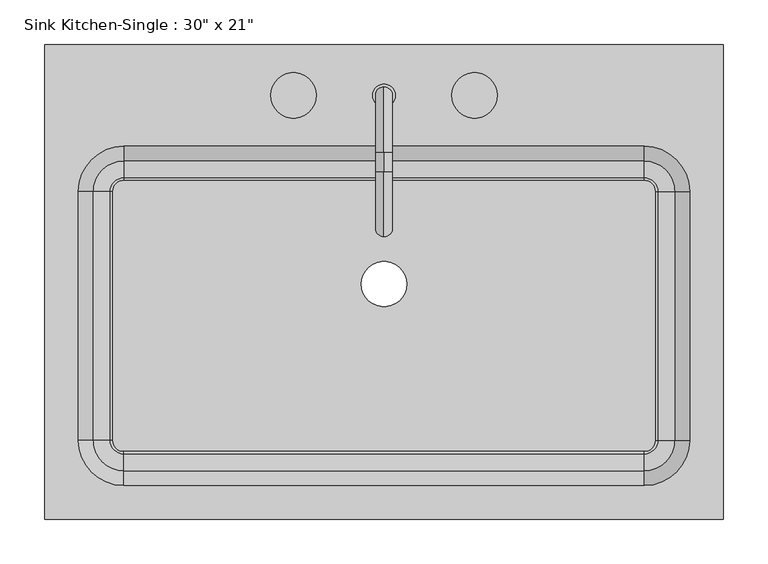
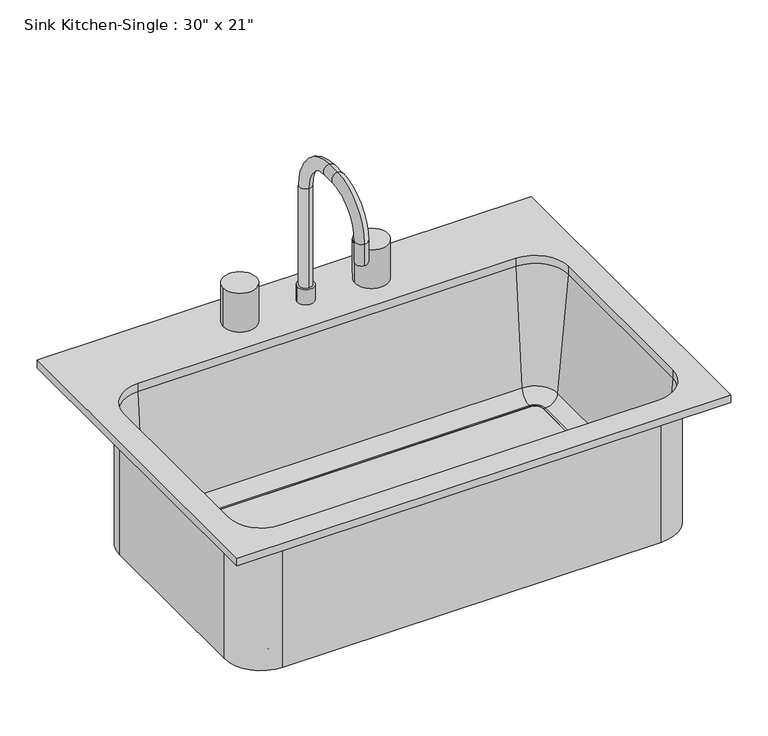
"""IFC4 building model written with IfcOpenShell, lengths in millimetres: flow terminal geometry."""

from ifc_helpers import new_model, si_unit, point, frame, frame_2d, origin, place, context, project, spatial, polyline, circle_curve, ellipse_curve, trimmed, segment, composite_curve, outline, extrude, source, transform, mapped, element, save
from ifc_brep_helpers import plane_surface, cylinder_surface, revolved_surface, advanced_brep


def flow_terminal_38af2918(model_context):
    return source(origin(), model_context, "Body", "SolidModel", [
        advanced_brep(
        [(396.6892406, 269.0454011, 927.1), (-365.3107594, 269.0454011, 927.1), (-365.3107594, -264.3545989, 927.1), (396.6892406, -264.3545989, 927.1), (307.7892406, 154.7454011, 927.1), (358.5892406, 103.9454011, 927.1), (358.5892406, -175.4545989, 927.1), (307.7892406, -226.2545989, 927.1), (-276.4107594, -226.2545989, 927.1), (-327.2107594, -175.4545989, 927.1), (-327.2107594, 103.9454011, 927.1), (-276.4107594, 154.7454011, 927.1), (396.6892406, 269.0454011, 914.4), (396.6892406, -264.3545989, 914.4), (-365.3107594, -264.3545989, 914.4), (-365.3107594, 269.0454011, 914.4), (364.9392406, 103.9454011, 914.4), (307.7892406, 161.0954011, 914.4), (-276.4107594, 161.0954011, 914.4), (-333.5607594, 103.9454011, 914.4), (-333.5607594, -175.4545989, 914.4), (-276.4107594, -232.6045989, 914.4), (307.7892406, -232.6045989, 914.4), (364.9392406, -175.4545989, 914.4), (307.7892406, 154.7454011, 914.4), (358.5892406, 103.9454011, 914.4), (358.5892406, -175.4545989, 914.4), (307.7892406, -226.2545989, 914.4), (-276.4107594, -226.2545989, 914.4), (-327.2107594, -175.4545989, 914.4), (-327.2107594, 103.9454011, 914.4), (-276.4107594, 154.7454011, 914.4), (364.9392406, 103.9454011, 698.5), (307.7892406, 161.0954011, 698.5), (320.4892406, 103.9454011, 698.5), (307.7892406, 116.6454011, 698.5), (320.4892406, 103.9454011, 708.025), (307.7892406, 116.6454011, 708.025), (323.0776588, 103.9454011, 708.025), (307.7892406, 119.2338193, 708.025), (342.0551678, 103.9454011, 725.4146831), (307.7892406, 138.2113283, 725.4146831), (364.9392406, -175.4545989, 698.5), (320.4892406, -175.4545989, 698.5), (320.4892406, -175.4545989, 708.025), (323.0776588, -175.4545989, 708.025), (342.0551678, -175.4545989, 725.4146831), (307.7892406, -232.6045989, 698.5), (307.7892406, -188.1545989, 698.5), (307.7892406, -188.1545989, 708.025), (307.7892406, -190.7430171, 708.025), (307.7892406, -209.7205261, 725.4146831), (-276.4107594, -232.6045989, 698.5), (-276.4107594, -188.1545989, 698.5), (-276.4107594, -188.1545989, 708.025), (-276.4107594, -190.7430171, 708.025), (-276.4107594, -209.7205261, 725.4146831), (-333.5607594, -175.4545989, 698.5), (-289.1107594, -175.4545989, 698.5), (-289.1107594, -175.4545989, 708.025), (-291.6991776, -175.4545989, 708.025), (-310.6766866, -175.4545989, 725.4146831), (-333.5607594, 103.9454011, 698.5), (-289.1107594, 103.9454011, 698.5), (-289.1107594, 103.9454011, 708.025), (-291.6991776, 103.9454011, 708.025), (-310.6766866, 103.9454011, 725.4146831), (-276.4107594, 161.0954011, 698.5), (-276.4107594, 116.6454011, 698.5), (-276.4107594, 116.6454011, 708.025), (-276.4107594, 119.2338193, 708.025), (-276.4107594, 138.2113283, 725.4146831)],
        [
            (0, 1),
            (1, 2),
            (2, 3),
            (3, 0),
            (4, 5, circle_curve(frame((307.7892406, 103.9454011, 927.1), z_axis=(0.0, 0.0, -1.0), x_axis=(1.0, 0.0, 0.0)), 50.8)),
            (5, 6),
            (6, 7, circle_curve(frame((307.7892406, -175.4545989, 927.1), z_axis=(0.0, 0.0, -1.0), x_axis=(1.0, 0.0, 0.0)), 50.8)),
            (7, 8),
            (8, 9, circle_curve(frame((-276.4107594, -175.4545989, 927.1), z_axis=(0.0, 0.0, -1.0), x_axis=(1.0, 0.0, 0.0)), 50.8)),
            (9, 10),
            (10, 11, circle_curve(frame((-276.4107594, 103.9454011, 927.1), z_axis=(0.0, 0.0, -1.0), x_axis=(1.0, 0.0, 0.0)), 50.8)),
            (11, 4),
            (12, 13),
            (13, 14),
            (14, 15),
            (15, 12),
            (16, 17, circle_curve(frame((307.7892406, 103.9454011, 914.4), z_axis=(0.0, 0.0, 1.0), x_axis=(0.0, 1.0, 0.0)), 57.15)),
            (17, 18),
            (18, 19, circle_curve(frame((-276.4107594, 103.9454011, 914.4), z_axis=(0.0, 0.0, 1.0), x_axis=(-1.0, 0.0, 0.0)), 57.15)),
            (19, 20),
            (20, 21, circle_curve(frame((-276.4107594, -175.4545989, 914.4), z_axis=(0.0, 0.0, 1.0), x_axis=(0.0, -1.0, 0.0)), 57.15)),
            (21, 22),
            (22, 23, circle_curve(frame((307.7892406, -175.4545989, 914.4), z_axis=(0.0, 0.0, 1.0), x_axis=(1.0, 0.0, 0.0)), 57.15)),
            (23, 16),
            (0, 12),
            (15, 1),
            (14, 2),
            (13, 3),
            (4, 24),
            (24, 25, circle_curve(frame((307.7892406, 103.9454011, 914.4), z_axis=(0.0, 0.0, -1.0), x_axis=(1.0, 0.0, 0.0)), 50.8)),
            (25, 5),
            (25, 26),
            (26, 6),
            (26, 27, circle_curve(frame((307.7892406, -175.4545989, 914.4), z_axis=(0.0, 0.0, -1.0), x_axis=(1.0, 0.0, 0.0)), 50.8)),
            (27, 7),
            (27, 28),
            (28, 8),
            (28, 29, circle_curve(frame((-276.4107594, -175.4545989, 914.4), z_axis=(0.0, 0.0, -1.0), x_axis=(1.0, 0.0, 0.0)), 50.8)),
            (29, 9),
            (29, 30),
            (30, 10),
            (30, 31, circle_curve(frame((-276.4107594, 103.9454011, 914.4), z_axis=(0.0, 0.0, -1.0), x_axis=(1.0, 0.0, 0.0)), 50.8)),
            (31, 11),
            (31, 24),
            (32, 33, circle_curve(frame((307.7892406, 103.9454011, 698.5), z_axis=(0.0, 0.0, 1.0), x_axis=(0.0, 1.0, 0.0)), 57.15)),
            (33, 17),
            (16, 32),
            (32, 34),
            (34, 35, circle_curve(frame((307.7892406, 103.9454011, 698.5), z_axis=(0.0, 0.0, 1.0), x_axis=(0.0, 1.0, 0.0)), 12.7)),
            (35, 33),
            (34, 36),
            (36, 37, circle_curve(frame((307.7892406, 103.9454011, 708.025), z_axis=(0.0, 0.0, 1.0), x_axis=(0.0, 1.0, 0.0)), 12.7)),
            (37, 35),
            (36, 38),
            (38, 39, circle_curve(frame((307.7892406, 103.9454011, 708.025), z_axis=(0.0, 0.0, 1.0), x_axis=(0.0, 1.0, 0.0)), 15.2884182)),
            (39, 37),
            (38, 40, circle_curve(frame((323.0776588, 103.9454011, 727.075), z_axis=(0.0, -1.0, 0.0), x_axis=(1.0, 0.0, 0.0)), 19.05)),
            (40, 41, circle_curve(frame((307.7892406, 103.9454011, 725.4146831), z_axis=(0.0, 0.0, 1.0), x_axis=(0.0, 1.0, 0.0)), 34.2659272)),
            (41, 39, circle_curve(frame((307.7892406, 119.2338193, 727.075), z_axis=(-1.0, 0.0, 0.0), x_axis=(0.0, 1.0, 0.0)), 19.05)),
            (40, 25),
            (24, 41),
            (23, 42),
            (42, 32),
            (42, 43),
            (43, 34),
            (43, 44),
            (44, 36),
            (44, 45),
            (45, 38),
            (45, 46, circle_curve(frame((323.0776588, -175.4545989, 727.075), z_axis=(0.0, -1.0, 0.0), x_axis=(1.0, 0.0, 0.0)), 19.05)),
            (46, 40),
            (46, 26),
            (22, 47),
            (47, 42, circle_curve(frame((307.7892406, -175.4545989, 698.5), z_axis=(0.0, 0.0, 1.0), x_axis=(1.0, 0.0, 0.0)), 57.15)),
            (47, 48),
            (48, 43, circle_curve(frame((307.7892406, -175.4545989, 698.5), z_axis=(0.0, 0.0, 1.0), x_axis=(1.0, 0.0, 0.0)), 12.7)),
            (48, 49),
            (49, 44, circle_curve(frame((307.7892406, -175.4545989, 708.025), z_axis=(0.0, 0.0, 1.0), x_axis=(1.0, 0.0, 0.0)), 12.7)),
            (49, 50),
            (50, 45, circle_curve(frame((307.7892406, -175.4545989, 708.025), z_axis=(0.0, 0.0, 1.0), x_axis=(1.0, 0.0, 0.0)), 15.2884182)),
            (50, 51, circle_curve(frame((307.7892406, -190.7430171, 727.075), z_axis=(-1.0, 0.0, 0.0), x_axis=(0.0, -1.0, 0.0)), 19.05)),
            (51, 46, circle_curve(frame((307.7892406, -175.4545989, 725.4146831), z_axis=(0.0, 0.0, 1.0), x_axis=(1.0, 0.0, 0.0)), 34.2659272)),
            (51, 27),
            (21, 52),
            (52, 47),
            (52, 53),
            (53, 48),
            (53, 54),
            (54, 49),
            (54, 55),
            (55, 50),
            (55, 56, circle_curve(frame((-276.4107594, -190.7430171, 727.075), z_axis=(-1.0, 0.0, 0.0), x_axis=(0.0, -1.0, 0.0)), 19.05)),
            (56, 51),
            (56, 28),
            (20, 57),
            (57, 52, circle_curve(frame((-276.4107594, -175.4545989, 698.5), z_axis=(0.0, 0.0, 1.0), x_axis=(0.0, -1.0, 0.0)), 57.15)),
            (57, 58),
            (58, 53, circle_curve(frame((-276.4107594, -175.4545989, 698.5), z_axis=(0.0, 0.0, 1.0), x_axis=(0.0, -1.0, 0.0)), 12.7)),
            (58, 59),
            (59, 54, circle_curve(frame((-276.4107594, -175.4545989, 708.025), z_axis=(0.0, 0.0, 1.0), x_axis=(0.0, -1.0, 0.0)), 12.7)),
            (59, 60),
            (60, 55, circle_curve(frame((-276.4107594, -175.4545989, 708.025), z_axis=(0.0, 0.0, 1.0), x_axis=(0.0, -1.0, 0.0)), 15.2884182)),
            (60, 61, circle_curve(frame((-291.6991776, -175.4545989, 727.075), z_axis=(0.0, 1.0, 0.0), x_axis=(-1.0, 0.0, 0.0)), 19.05)),
            (61, 56, circle_curve(frame((-276.4107594, -175.4545989, 725.4146831), z_axis=(0.0, 0.0, 1.0), x_axis=(0.0, -1.0, 0.0)), 34.2659272)),
            (61, 29),
            (19, 62),
            (62, 57),
            (62, 63),
            (63, 58),
            (63, 64),
            (64, 59),
            (64, 65),
            (65, 60),
            (65, 66, circle_curve(frame((-291.6991776, 103.9454011, 727.075), z_axis=(0.0, 1.0, 0.0), x_axis=(-1.0, 0.0, 0.0)), 19.05)),
            (66, 61),
            (66, 30),
            (18, 67),
            (67, 62, circle_curve(frame((-276.4107594, 103.9454011, 698.5), z_axis=(0.0, 0.0, 1.0), x_axis=(-1.0, 0.0, 0.0)), 57.15)),
            (67, 68),
            (68, 63, circle_curve(frame((-276.4107594, 103.9454011, 698.5), z_axis=(0.0, 0.0, 1.0), x_axis=(-1.0, 0.0, 0.0)), 12.7)),
            (68, 69),
            (69, 64, circle_curve(frame((-276.4107594, 103.9454011, 708.025), z_axis=(0.0, 0.0, 1.0), x_axis=(-1.0, 0.0, 0.0)), 12.7)),
            (69, 70),
            (70, 65, circle_curve(frame((-276.4107594, 103.9454011, 708.025), z_axis=(0.0, 0.0, 1.0), x_axis=(-1.0, 0.0, 0.0)), 15.2884182)),
            (70, 71, circle_curve(frame((-276.4107594, 119.2338193, 727.075), z_axis=(1.0, 0.0, 0.0), x_axis=(0.0, 1.0, 0.0)), 19.05)),
            (71, 66, circle_curve(frame((-276.4107594, 103.9454011, 725.4146831), z_axis=(0.0, 0.0, 1.0), x_axis=(-1.0, 0.0, 0.0)), 34.2659272)),
            (71, 31),
            (33, 67),
            (35, 68),
            (37, 69),
            (39, 70),
            (41, 71),
        ],
        [
            plane_surface(frame((-365.3107594, 269.0454011, 927.1), z_axis=(0.0, 0.0, 1.0), x_axis=(-1.0, 0.0, 0.0))),
            plane_surface(frame((-365.3107594, 269.0454011, 914.4), z_axis=(0.0, 0.0, -1.0), x_axis=(1.0, 0.0, 0.0))),
            plane_surface(frame((396.6892406, 269.0454011, 927.1), z_axis=(0.0, 1.0, 0.0), x_axis=(0.0, 0.0, -1.0))),
            plane_surface(frame((-365.3107594, 269.0454011, 927.1), z_axis=(-1.0, 0.0, 0.0), x_axis=(0.0, 0.0, -1.0))),
            plane_surface(frame((-365.3107594, -264.3545989, 927.1), z_axis=(0.0, -1.0, 0.0), x_axis=(0.0, 0.0, -1.0))),
            plane_surface(frame((396.6892406, -264.3545989, 927.1), z_axis=(1.0, 0.0, 0.0), x_axis=(0.0, 0.0, -1.0))),
            revolved_surface(polyline([(358.58924060000004, 103.9454011, 914.4), (358.58924060000004, 103.9454011, 927.1)]), (307.7892406, 103.9454011, 0.0), (0.0, 0.0, -1.0)),
            plane_surface(frame((358.5892406, 103.9454011, 927.1), z_axis=(-1.0, 0.0, 0.0), x_axis=(0.0, 0.0, -1.0))),
            revolved_surface(polyline([(358.58924060000004, -175.4545989, 914.4), (358.58924060000004, -175.4545989, 927.1)]), (307.7892406, -175.4545989, 0.0), (0.0, 0.0, -1.0)),
            plane_surface(frame((307.7892406, -226.2545989, 927.1), z_axis=(0.0, 1.0, 0.0), x_axis=(0.0, 0.0, -1.0))),
            revolved_surface(polyline([(-225.6107594, -175.4545989, 914.4), (-225.6107594, -175.4545989, 927.1)]), (-276.4107594, -175.4545989, 0.0), (0.0, 0.0, -1.0)),
            plane_surface(frame((-327.2107594, -175.4545989, 927.1), z_axis=(1.0, 0.0, 0.0), x_axis=(0.0, 0.0, -1.0))),
            revolved_surface(polyline([(-225.6107594, 103.9454011, 914.4), (-225.6107594, 103.9454011, 927.1)]), (-276.4107594, 103.9454011, 0.0), (0.0, 0.0, -1.0)),
            plane_surface(frame((-276.4107594, 154.7454011, 927.1), z_axis=(0.0, -1.0, 0.0), x_axis=(0.0, 0.0, -1.0))),
            cylinder_surface(frame((307.7892406, 103.9454011, 0.0), z_axis=(0.0, 0.0, -1.0), x_axis=(0.0, 1.0, 0.0)), 57.15),
            plane_surface(frame((307.7892406, 103.9454011, 698.5), z_axis=(0.0, 0.0, -1.0), x_axis=(0.0, 1.0, 0.0))),
            revolved_surface(polyline([(307.7892406, 116.6454011, 698.5), (307.7892406, 116.6454011, 708.025)]), (307.7892406, 103.9454011, 0.0), (0.0, 0.0, -1.0)),
            plane_surface(frame((307.7892406, 103.9454011, 708.025), z_axis=(0.0, 0.0, 1.0), x_axis=(0.0, 1.0, 0.0))),
            revolved_surface(trimmed(ellipse_curve(frame((307.7892406, 119.2338193, 727.075), z_axis=(1.0, 0.0, 0.0), x_axis=(0.0, 1.0, 0.0)), 19.05, 19.05), [point((307.7892406, 119.2338193, 708.025))], [point((307.7892406, 138.2113283, 725.4146831))], True, "CARTESIAN"), (307.7892406, 103.9454011, 0.0), (0.0, 0.0, -1.0)),
            revolved_surface(polyline([(307.7892406, 138.2113283, 725.4146831), (307.7892406, 154.7454011, 914.4)]), (307.7892406, 103.9454011, 0.0), (0.0, 0.0, -1.0)),
            plane_surface(frame((364.9392406, 103.9454011, 914.4), z_axis=(1.0, 0.0, 0.0), x_axis=(0.0, -1.0, 0.0))),
            plane_surface(frame((364.9392406, 103.9454011, 698.5), z_axis=(0.0, 0.0, -1.0), x_axis=(0.0, -1.0, 0.0))),
            plane_surface(frame((320.4892406, 103.9454011, 698.5), z_axis=(-1.0, 0.0, 0.0), x_axis=(0.0, -1.0, 0.0))),
            plane_surface(frame((320.4892406, 103.9454011, 708.025), z_axis=(0.0, 0.0, 1.0), x_axis=(0.0, -1.0, 0.0))),
            revolved_surface(polyline([(342.1276588, -175.45459889999998, 727.075), (342.1276588, 103.9454011, 727.075)]), (323.0776588, 103.9454011, 727.075), (0.0, -1.0, 0.0)),
            plane_surface(frame((342.0551678, 103.9454011, 725.4146831), z_axis=(-0.9961946980917442, 0.0, 0.08715574274767306), x_axis=(0.0, -1.0, 0.0))),
            cylinder_surface(frame((307.7892406, -175.4545989, 0.0), z_axis=(0.0, 0.0, -1.0), x_axis=(1.0, 0.0, 0.0)), 57.15),
            plane_surface(frame((307.7892406, -175.4545989, 698.5), z_axis=(0.0, 0.0, -1.0), x_axis=(1.0, 0.0, 0.0))),
            revolved_surface(polyline([(320.4892406, -175.4545989, 698.5), (320.4892406, -175.4545989, 708.025)]), (307.7892406, -175.4545989, 0.0), (0.0, 0.0, -1.0)),
            plane_surface(frame((307.7892406, -175.4545989, 708.025), z_axis=(0.0, 0.0, 1.0), x_axis=(1.0, 0.0, 0.0))),
            revolved_surface(trimmed(ellipse_curve(frame((323.0776588, -175.4545989, 727.075), z_axis=(0.0, -1.0, 0.0), x_axis=(1.0, 0.0, 0.0)), 19.05, 19.05), [point((323.0776588, -175.4545989, 708.025))], [point((342.0551678, -175.4545989, 725.4146831))], True, "CARTESIAN"), (307.7892406, -175.4545989, 0.0), (0.0, 0.0, -1.0)),
            revolved_surface(polyline([(342.0551678, -175.4545989, 725.4146831), (358.5892406, -175.4545989, 914.4)]), (307.7892406, -175.4545989, 0.0), (0.0, 0.0, -1.0)),
            plane_surface(frame((307.7892406, -232.6045989, 914.4), z_axis=(0.0, -1.0, 0.0), x_axis=(-1.0, 0.0, 0.0))),
            plane_surface(frame((307.7892406, -232.6045989, 698.5), z_axis=(0.0, 0.0, -1.0), x_axis=(-1.0, 0.0, 0.0))),
            plane_surface(frame((307.7892406, -188.1545989, 698.5), z_axis=(0.0, 1.0, 0.0), x_axis=(-1.0, 0.0, 0.0))),
            plane_surface(frame((307.7892406, -188.1545989, 708.025), z_axis=(0.0, 0.0, 1.0), x_axis=(-1.0, 0.0, 0.0))),
            revolved_surface(polyline([(-276.4107594, -209.79301710000001, 727.075), (307.7892406, -209.79301710000001, 727.075)]), (307.7892406, -190.7430171, 727.075), (-1.0, 0.0, 0.0)),
            plane_surface(frame((307.7892406, -209.7205261, 725.4146831), z_axis=(0.0, 0.9961946980917442, 0.08715574274767306), x_axis=(-1.0, 0.0, 0.0))),
            cylinder_surface(frame((-276.4107594, -175.4545989, 0.0), z_axis=(0.0, 0.0, -1.0), x_axis=(0.0, -1.0, 0.0)), 57.15),
            plane_surface(frame((-276.4107594, -175.4545989, 698.5), z_axis=(0.0, 0.0, -1.0), x_axis=(0.0, -1.0, 0.0))),
            revolved_surface(polyline([(-276.4107594, -188.1545989, 698.5), (-276.4107594, -188.1545989, 708.025)]), (-276.4107594, -175.4545989, 0.0), (0.0, 0.0, -1.0)),
            plane_surface(frame((-276.4107594, -175.4545989, 708.025), z_axis=(0.0, 0.0, 1.0), x_axis=(0.0, -1.0, 0.0))),
            revolved_surface(trimmed(ellipse_curve(frame((-276.4107594, -190.7430171, 727.075), z_axis=(-1.0, 0.0, 0.0), x_axis=(0.0, -1.0, 0.0)), 19.05, 19.05), [point((-276.4107594, -190.7430171, 708.025))], [point((-276.4107594, -209.7205261, 725.4146831))], True, "CARTESIAN"), (-276.4107594, -175.4545989, 0.0), (0.0, 0.0, -1.0)),
            revolved_surface(polyline([(-276.4107594, -209.7205261, 725.4146831), (-276.4107594, -226.2545989, 914.4)]), (-276.4107594, -175.4545989, 0.0), (0.0, 0.0, -1.0)),
            plane_surface(frame((-333.5607594, -175.4545989, 914.4), z_axis=(-1.0, 0.0, 0.0), x_axis=(0.0, 1.0, 0.0))),
            plane_surface(frame((-333.5607594, -175.4545989, 698.5), z_axis=(0.0, 0.0, -1.0), x_axis=(0.0, 1.0, 0.0))),
            plane_surface(frame((-289.1107594, -175.4545989, 698.5), z_axis=(1.0, 0.0, 0.0), x_axis=(0.0, 1.0, 0.0))),
            plane_surface(frame((-289.1107594, -175.4545989, 708.025), z_axis=(0.0, 0.0, 1.0), x_axis=(0.0, 1.0, 0.0))),
            revolved_surface(polyline([(-310.7491776, 103.94540109999997, 727.075), (-310.7491776, -175.4545989, 727.075)]), (-291.6991776, -175.4545989, 727.075), (0.0, 1.0, 0.0)),
            plane_surface(frame((-310.6766866, -175.4545989, 725.4146831), z_axis=(0.9961946980917442, 0.0, 0.08715574274767306), x_axis=(0.0, 1.0, 0.0))),
            cylinder_surface(frame((-276.4107594, 103.9454011, 0.0), z_axis=(0.0, 0.0, -1.0), x_axis=(-1.0, 0.0, 0.0)), 57.15),
            plane_surface(frame((-276.4107594, 103.9454011, 698.5), z_axis=(0.0, 0.0, -1.0), x_axis=(-1.0, 0.0, 0.0))),
            revolved_surface(polyline([(-289.1107594, 103.9454011, 698.5), (-289.1107594, 103.9454011, 708.025)]), (-276.4107594, 103.9454011, 0.0), (0.0, 0.0, -1.0)),
            plane_surface(frame((-276.4107594, 103.9454011, 708.025), z_axis=(0.0, 0.0, 1.0), x_axis=(-1.0, 0.0, 0.0))),
            revolved_surface(trimmed(ellipse_curve(frame((-291.6991776, 103.9454011, 727.075), z_axis=(0.0, 1.0, 0.0), x_axis=(-1.0, 0.0, 0.0)), 19.05, 19.05), [point((-291.6991776, 103.9454011, 708.025))], [point((-310.6766866, 103.9454011, 725.4146831))], True, "CARTESIAN"), (-276.4107594, 103.9454011, 0.0), (0.0, 0.0, -1.0)),
            revolved_surface(polyline([(-310.6766866, 103.9454011, 725.4146831), (-327.2107594, 103.9454011, 914.4)]), (-276.4107594, 103.9454011, 0.0), (0.0, 0.0, -1.0)),
            plane_surface(frame((-276.4107594, 161.0954011, 914.4), z_axis=(0.0, 1.0, 0.0), x_axis=(1.0, 0.0, 0.0))),
            plane_surface(frame((-276.4107594, 161.0954011, 698.5), z_axis=(0.0, 0.0, -1.0), x_axis=(1.0, 0.0, 0.0))),
            plane_surface(frame((-276.4107594, 116.6454011, 698.5), z_axis=(0.0, -1.0, 0.0), x_axis=(1.0, 0.0, 0.0))),
            plane_surface(frame((-276.4107594, 116.6454011, 708.025), z_axis=(0.0, 0.0, 1.0), x_axis=(1.0, 0.0, 0.0))),
            revolved_surface(polyline([(307.7892406, 138.2838193, 727.075), (-276.4107594, 138.2838193, 727.075)]), (-276.4107594, 119.2338193, 727.075), (1.0, 0.0, 0.0)),
            plane_surface(frame((-276.4107594, 138.2113283, 725.4146831), z_axis=(0.0, -0.9961946980917442, 0.08715574274767306), x_axis=(1.0, 0.0, 0.0))),
        ],
        [
            (0, [[1, 2, 3, 4], [5, 6, 7, 8, 9, 10, 11, 12]]),
            (1, [[13, 14, 15, 16], [17, 18, 19, 20, 21, 22, 23, 24]]),
            (2, [[-1, 25, -16, 26]]),
            (3, [[-2, -26, -15, 27]]),
            (4, [[-3, -27, -14, 28]]),
            (5, [[-4, -28, -13, -25]]),
            (6, [[-5, 29, 30, 31]]),
            (7, [[-6, -31, 32, 33]]),
            (8, [[-7, -33, 34, 35]]),
            (9, [[-8, -35, 36, 37]]),
            (10, [[-9, -37, 38, 39]]),
            (11, [[-10, -39, 40, 41]]),
            (12, [[-11, -41, 42, 43]]),
            (13, [[-12, -43, 44, -29]]),
            (14, [[45, 46, -17, 47]]),
            (15, [[-45, 48, 49, 50]]),
            (16, [[-49, 51, 52, 53]]),
            (17, [[-52, 54, 55, 56]]),
            (18, [[-55, 57, 58, 59]]),
            (19, [[-58, 60, -30, 61]]),
            (20, [[-47, -24, 62, 63]]),
            (21, [[-48, -63, 64, 65]]),
            (22, [[-51, -65, 66, 67]]),
            (23, [[-54, -67, 68, 69]]),
            (24, [[-57, -69, 70, 71]]),
            (25, [[-60, -71, 72, -32]]),
            (26, [[-62, -23, 73, 74]]),
            (27, [[-64, -74, 75, 76]]),
            (28, [[-66, -76, 77, 78]]),
            (29, [[-68, -78, 79, 80]]),
            (30, [[-70, -80, 81, 82]]),
            (31, [[-72, -82, 83, -34]]),
            (32, [[-73, -22, 84, 85]]),
            (33, [[-75, -85, 86, 87]]),
            (34, [[-77, -87, 88, 89]]),
            (35, [[-79, -89, 90, 91]]),
            (36, [[-81, -91, 92, 93]]),
            (37, [[-83, -93, 94, -36]]),
            (38, [[-84, -21, 95, 96]]),
            (39, [[-86, -96, 97, 98]]),
            (40, [[-88, -98, 99, 100]]),
            (41, [[-90, -100, 101, 102]]),
            (42, [[-92, -102, 103, 104]]),
            (43, [[-94, -104, 105, -38]]),
            (44, [[-95, -20, 106, 107]]),
            (45, [[-97, -107, 108, 109]]),
            (46, [[-99, -109, 110, 111]]),
            (47, [[-101, -111, 112, 113]]),
            (48, [[-103, -113, 114, 115]]),
            (49, [[-105, -115, 116, -40]]),
            (50, [[-106, -19, 117, 118]]),
            (51, [[-108, -118, 119, 120]]),
            (52, [[-110, -120, 121, 122]]),
            (53, [[-112, -122, 123, 124]]),
            (54, [[-114, -124, 125, 126]]),
            (55, [[-116, -126, 127, -42]]),
            (56, [[-46, 128, -117, -18]]),
            (57, [[-50, 129, -119, -128]]),
            (58, [[-53, 130, -121, -129]]),
            (59, [[-56, 131, -123, -130]]),
            (60, [[-59, 132, -125, -131]]),
            (61, [[-61, -44, -127, -132]]),
        ],
    ),
        advanced_brep(
        [(2.9892406, 211.8954011, 927.1), (28.3892406, 211.8954011, 927.1), (15.6892406, 221.4204011, 1114.425), (15.6892406, 202.3704011, 1114.425), (15.6892406, 202.3704011, 952.5), (15.6892406, 221.4204011, 952.5), (15.6892406, 148.3954011, 1187.45), (15.6892406, 148.3954011, 1168.4), (15.6892406, 126.1704011, 1187.45), (15.6892406, 126.1704011, 1168.4), (15.6892406, 53.1454011, 1114.425), (15.6892406, 72.1954011, 1114.425), (15.6892406, 53.1454011, 1079.5), (15.6892406, 72.1954011, 1079.5), (2.9892406, 211.8954011, 952.5), (28.3892406, 211.8954011, 952.5)],
        [
            (0, 1, circle_curve(frame((15.6892406, 211.8954011, 927.1), z_axis=(0.0, 0.0, -1.0), x_axis=(1.0, 0.0, 0.0)), 12.7)),
            (1, 0, circle_curve(frame((15.6892406, 211.8954011, 927.1), z_axis=(0.0, 0.0, -1.0), x_axis=(1.0, 0.0, 0.0)), 12.7)),
            (2, 3, circle_curve(frame((15.6892406, 211.8954011, 1114.425), z_axis=(0.0, 0.0, -1.0), x_axis=(0.0, -1.0, 0.0)), 9.525)),
            (3, 4),
            (4, 5, circle_curve(frame((15.6892406, 211.8954011, 952.5), z_axis=(0.0, 0.0, 1.0), x_axis=(0.0, -1.0, 0.0)), 9.525)),
            (5, 2),
            (3, 2, circle_curve(frame((15.6892406, 211.8954011, 1114.425), z_axis=(0.0, 0.0, -1.0), x_axis=(0.0, -1.0, 0.0)), 9.525)),
            (5, 4, circle_curve(frame((15.6892406, 211.8954011, 952.5), z_axis=(0.0, 0.0, 1.0), x_axis=(0.0, -1.0, 0.0)), 9.525)),
            (2, 6, circle_curve(frame((15.6892406, 148.3954011, 1114.425), z_axis=(1.0, 0.0, 0.0), x_axis=(0.0, 1.0, 0.0)), 73.025)),
            (6, 7, circle_curve(frame((15.6892406, 148.3954011, 1177.925), z_axis=(0.0, 1.0, 0.0), x_axis=(0.0, 0.0, -1.0)), 9.525)),
            (7, 3, circle_curve(frame((15.6892406, 148.3954011, 1114.425), z_axis=(-1.0, 0.0, 0.0), x_axis=(0.0, 1.0, 0.0)), 53.975)),
            (7, 6, circle_curve(frame((15.6892406, 148.3954011, 1177.925), z_axis=(0.0, 1.0, 0.0), x_axis=(0.0, 0.0, -1.0)), 9.525)),
            (6, 8),
            (8, 9, circle_curve(frame((15.6892406, 126.1704011, 1177.925), z_axis=(0.0, 1.0, 0.0), x_axis=(0.0, 0.0, -1.0)), 9.525)),
            (9, 7),
            (9, 8, circle_curve(frame((15.6892406, 126.1704011, 1177.925), z_axis=(0.0, 1.0, 0.0), x_axis=(0.0, 0.0, -1.0)), 9.525)),
            (8, 10, circle_curve(frame((15.6892406, 126.1704011, 1114.425), z_axis=(1.0, 0.0, 0.0), x_axis=(0.0, 0.0, 1.0)), 73.025)),
            (10, 11, circle_curve(frame((15.6892406, 62.6704011, 1114.425), z_axis=(0.0, 0.0, 1.0), x_axis=(0.0, 1.0, 0.0)), 9.525)),
            (11, 9, circle_curve(frame((15.6892406, 126.1704011, 1114.425), z_axis=(-1.0, 0.0, 0.0), x_axis=(0.0, 0.0, 1.0)), 53.975)),
            (11, 10, circle_curve(frame((15.6892406, 62.6704011, 1114.425), z_axis=(0.0, 0.0, 1.0), x_axis=(0.0, 1.0, 0.0)), 9.525)),
            (12, 13, circle_curve(frame((15.6892406, 62.6704011, 1079.5), z_axis=(0.0, 0.0, -1.0), x_axis=(0.0, 1.0, 0.0)), 9.525)),
            (13, 12, circle_curve(frame((15.6892406, 62.6704011, 1079.5), z_axis=(0.0, 0.0, -1.0), x_axis=(0.0, 1.0, 0.0)), 9.525)),
            (10, 12),
            (13, 11),
            (14, 15, circle_curve(frame((15.6892406, 211.8954011, 952.5), z_axis=(0.0, 0.0, 1.0), x_axis=(1.0, 0.0, 0.0)), 12.7)),
            (15, 14, circle_curve(frame((15.6892406, 211.8954011, 952.5), z_axis=(0.0, 0.0, 1.0), x_axis=(1.0, 0.0, 0.0)), 12.7)),
            (14, 0),
            (1, 15),
        ],
        [
            plane_surface(frame((15.6892406, 202.3704011, 927.1), z_axis=(0.0, 0.0, -1.0), x_axis=(1.0, 0.0, 0.0))),
            cylinder_surface(frame((15.6892406, 211.8954011, 927.1), z_axis=(0.0, 0.0, -1.0), x_axis=(0.0, -1.0, 0.0)), 9.525),
            revolved_surface(trimmed(ellipse_curve(frame((15.6892406, 211.8954011, 1114.425), z_axis=(0.0, 0.0, -1.0), x_axis=(0.0, -1.0, 0.0)), 9.525, 9.525), [point((15.6892406, 221.4204011, 1114.425))], [point((15.6892406, 202.3704011, 1114.425))], True, "CARTESIAN"), (15.6892406, 148.3954011, 1114.425), (1.0, 0.0, 0.0)),
            revolved_surface(trimmed(ellipse_curve(frame((15.6892406, 211.8954011, 1114.425), z_axis=(0.0, 0.0, -1.0), x_axis=(0.0, -1.0, 0.0)), 9.525, 9.525), [point((15.6892406, 202.3704011, 1114.425))], [point((15.6892406, 221.4204011, 1114.425))], True, "CARTESIAN"), (15.6892406, 148.3954011, 1114.425), (1.0, 0.0, 0.0)),
            cylinder_surface(frame((15.6892406, 148.3954011, 1177.925), z_axis=(0.0, 1.0, 0.0), x_axis=(0.0, 0.0, -1.0)), 9.525),
            revolved_surface(trimmed(ellipse_curve(frame((15.6892406, 126.1704011, 1177.925), z_axis=(0.0, 1.0, 0.0), x_axis=(0.0, 0.0, -1.0)), 9.525, 9.525), [point((15.6892406, 126.1704011, 1187.45))], [point((15.6892406, 126.1704011, 1168.4))], True, "CARTESIAN"), (15.6892406, 126.1704011, 1114.425), (1.0, 0.0, 0.0)),
            revolved_surface(trimmed(ellipse_curve(frame((15.6892406, 126.1704011, 1177.925), z_axis=(0.0, 1.0, 0.0), x_axis=(0.0, 0.0, -1.0)), 9.525, 9.525), [point((15.6892406, 126.1704011, 1168.4))], [point((15.6892406, 126.1704011, 1187.45))], True, "CARTESIAN"), (15.6892406, 126.1704011, 1114.425), (1.0, 0.0, 0.0)),
            plane_surface(frame((15.6892406, 53.1454011, 1079.5), z_axis=(0.0, 0.0, -1.0), x_axis=(-1.0, 0.0, 0.0))),
            cylinder_surface(frame((15.6892406, 62.6704011, 1114.425), z_axis=(0.0, 0.0, 1.0), x_axis=(0.0, 1.0, 0.0)), 9.525),
            plane_surface(frame((28.3892406, 211.8954011, 952.5), z_axis=(0.0, 0.0, 1.0), x_axis=(0.0, 1.0, 0.0))),
            cylinder_surface(frame((15.6892406, 211.8954011, 927.1), z_axis=(0.0, 0.0, 1.0), x_axis=(1.0, 0.0, 0.0)), 12.7),
        ],
        [
            (0, [[1, 2]]),
            (1, [[3, 4, 5, 6]]),
            (1, [[7, -6, 8, -4]]),
            (2, [[-3, 9, 10, 11]]),
            (3, [[-7, -11, 12, -9]]),
            (4, [[-10, 13, 14, 15]]),
            (4, [[-12, -15, 16, -13]]),
            (5, [[-14, 17, 18, 19]]),
            (6, [[-16, -19, 20, -17]]),
            (7, [[21, 22]]),
            (8, [[-18, 23, -22, 24]]),
            (8, [[-20, -24, -21, -23]]),
            (9, [[25, 26], [-5, -8]]),
            (10, [[-25, 27, -2, 28]]),
            (10, [[-26, -28, -1, -27]]),
        ],
    ),
        extrude(outline(composite_curve([segment(trimmed(circle_curve(frame_2d((-85.9107594, 211.8954011)), 25.4), [point((-111.3107594, 211.8954011))], [point((-60.5107594, 211.8954011))], False, "CARTESIAN"), True, "CONTINUOUS"), segment(trimmed(circle_curve(frame_2d((-85.9107594, 211.8954011)), 25.4), [point((-60.5107594, 211.8954011))], [point((-111.3107594, 211.8954011))], False, "CARTESIAN"), True, "CONTINUOUS")], self_intersect=False)), frame((0.0, 0.0, 927.1), z_axis=(0.0, 0.0, 1.0), x_axis=(1.0, 0.0, 0.0)), (0.0, 0.0, 1.0), 63.5),
        extrude(outline(composite_curve([segment(trimmed(circle_curve(frame_2d((117.2892406, 211.8954011)), 25.4), [point((91.8892406, 211.8954011))], [point((142.6892406, 211.8954011))], False, "CARTESIAN"), True, "CONTINUOUS"), segment(trimmed(circle_curve(frame_2d((117.2892406, 211.8954011)), 25.4), [point((142.6892406, 211.8954011))], [point((91.8892406, 211.8954011))], False, "CARTESIAN"), True, "CONTINUOUS")], self_intersect=False)), frame((0.0, 0.0, 927.1), z_axis=(0.0, 0.0, 1.0), x_axis=(1.0, 0.0, 0.0)), (0.0, 0.0, 1.0), 63.5),
        extrude(outline(composite_curve([segment(trimmed(circle_curve(frame_2d((307.7892406, 103.9454011)), 12.7), [point((307.7892406, 116.6454011))], [point((320.4892406, 103.9454011))], False, "CARTESIAN"), True, "CONTINUOUS"), segment(polyline([(320.4892406, 103.9454011), (320.4892406, -175.4545989)]), True, "CONTINUOUS"), segment(trimmed(circle_curve(frame_2d((307.7892406, -175.4545989)), 12.7), [point((320.4892406, -175.4545989))], [point((307.7892406, -188.1545989))], False, "CARTESIAN"), True, "CONTINUOUS"), segment(polyline([(307.7892406, -188.1545989), (-276.4107594, -188.1545989)]), True, "CONTINUOUS"), segment(trimmed(circle_curve(frame_2d((-276.4107594, -175.4545989)), 12.7), [point((-276.4107594, -188.1545989))], [point((-289.1107594, -175.4545989))], False, "CARTESIAN"), True, "CONTINUOUS"), segment(polyline([(-289.1107594, -175.4545989), (-289.1107594, 103.9454011)]), True, "CONTINUOUS"), segment(trimmed(circle_curve(frame_2d((-276.4107594, 103.9454011)), 12.7), [point((-289.1107594, 103.9454011))], [point((-276.4107594, 116.6454011))], False, "CARTESIAN"), True, "CONTINUOUS"), segment(polyline([(-276.4107594, 116.6454011), (307.7892406, 116.6454011)]), True, "CONTINUOUS")], self_intersect=False), holes=[composite_curve([segment(trimmed(circle_curve(frame_2d((15.6892406, 0.0)), 25.4), [point((-9.7107594, 0.0))], [point((41.0892406, 0.0))], True, "CARTESIAN"), True, "CONTINUOUS"), segment(trimmed(circle_curve(frame_2d((15.6892406, 0.0)), 25.4), [point((41.0892406, 0.0))], [point((-9.7107594, 0.0))], True, "CARTESIAN"), True, "CONTINUOUS")], self_intersect=False)]), frame((0.0, 0.0, 698.5), z_axis=(0.0, 0.0, 1.0), x_axis=(1.0, 0.0, 0.0)), (0.0, 0.0, 1.0), 9.525),
    ])


if __name__ == "__main__":
    model = new_model("IFC4")
    model_context = context("Model", 3, world=origin())
    ifc_project = project(units=[si_unit("LENGTHUNIT", "METRE", prefix="MILLI")], contexts=[model_context])
    site = spatial("IfcSite", under=ifc_project)
    building = spatial("IfcBuilding", under=site)
    placement = place(None, origin())
    flow_terminal_shape = flow_terminal_38af2918(model_context)
    element("IfcFlowTerminal", 1, ObjectType="Sink Kitchen-Single : 30\" x 21\"", at=placement, inside=building, context=model_context, shape_type="MappedRepresentation", body=[
        mapped(flow_terminal_shape, transform((0.0, 0.0, 0.0), x_axis=(1.0, 0.0, 0.0), y_axis=(0.0, 1.0, 0.0), z_axis=(0.0, 0.0, 1.0))),
    ])
    save(model, "model.ifc")

# Revit data of these elements
# Type "Sink Kitchen-Single : 30\" x 21\""
#   Assembly Code = "D2010410"
#   Counter Height = 3' - 0"
#   Depth = 1' - 9"
#   Width = 2' - 6"
#   Faucet Material = Steel, Polished
#   Sink Material = Steel, Polished
# Element 1 (IfcFlowTerminal, "Sink Kitchen-Single : 30\" x 21\"")
#   Materials on its faces: "Steel, Polished"
# Materials
#   "Steel, Polished": class "Metal", colour RGB 57 57 57, transparency 0, Description = "Polished steel", Cost = 0
